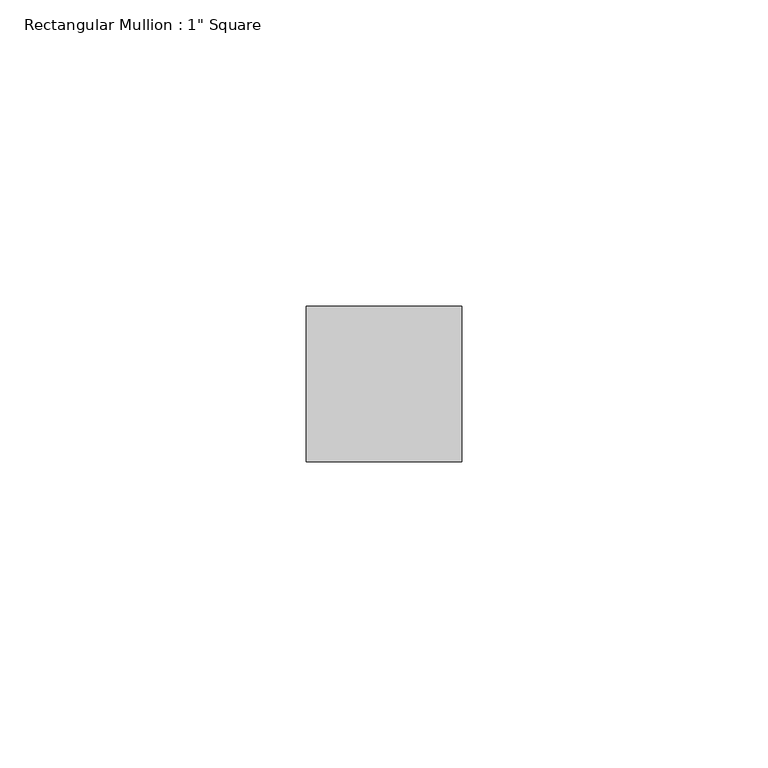
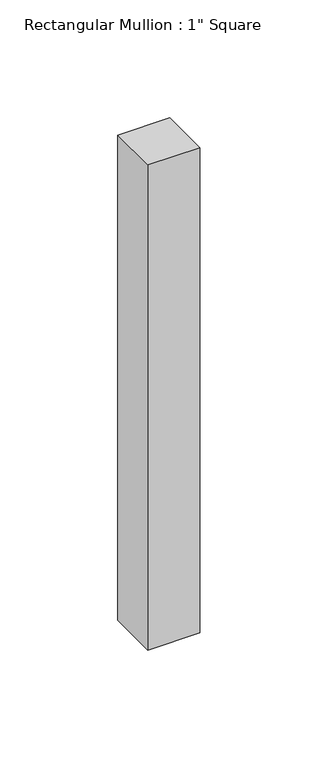
"""IFC4 building model written with IfcOpenShell, lengths in millimetres: member geometry."""

from ifc_helpers import new_model, si_unit, frame, origin, place, context, project, spatial, polyline, outline, extrude, source, transform, mapped, element, save


def member_b7a731ef(model_context):
    return source(origin(), model_context, "Body", "SweptSolid", [
        extrude(outline(polyline([(0.0, 12.7), (0.0, -12.7), (-25.4, -12.7), (-25.4, 12.7), (0.0, 12.7)])), frame((0.0, 0.0, -251.1186703), z_axis=(0.0, 0.0, 1.0), x_axis=(1.0, 0.0, 0.0)), (0.0, 0.0, 1.0), 251.1186703),
    ])


if __name__ == "__main__":
    model = new_model("IFC4")
    model_context = context("Model", 3, world=origin())
    ifc_project = project(units=[si_unit("LENGTHUNIT", "METRE", prefix="MILLI")], contexts=[model_context])
    site = spatial("IfcSite", under=ifc_project)
    building = spatial("IfcBuilding", under=site)
    placement = place(None, origin())
    member_shape = member_b7a731ef(model_context)
    element("IfcMember", 1, ObjectType="Rectangular Mullion : 1\" Square", at=placement, inside=building, context=model_context, shape_type="MappedRepresentation", body=[
        mapped(member_shape, transform((0.0, 0.0, 0.0), x_axis=(1.0, 0.0, 0.0), y_axis=(0.0, 1.0, 0.0), z_axis=(0.0, 0.0, 1.0))),
    ])
    save(model, "model.ifc")

# Revit data of these elements
# Type "Rectangular Mullion : 1\" Square"
#   built-in parameter 1007304 = 0.0833333 (stored number, unit not read)
#   built-in parameter 1007301 = 0.0416667 (stored number, unit not read)
#   built-in parameter 1007300 = 0.0416667 (stored number, unit not read)
